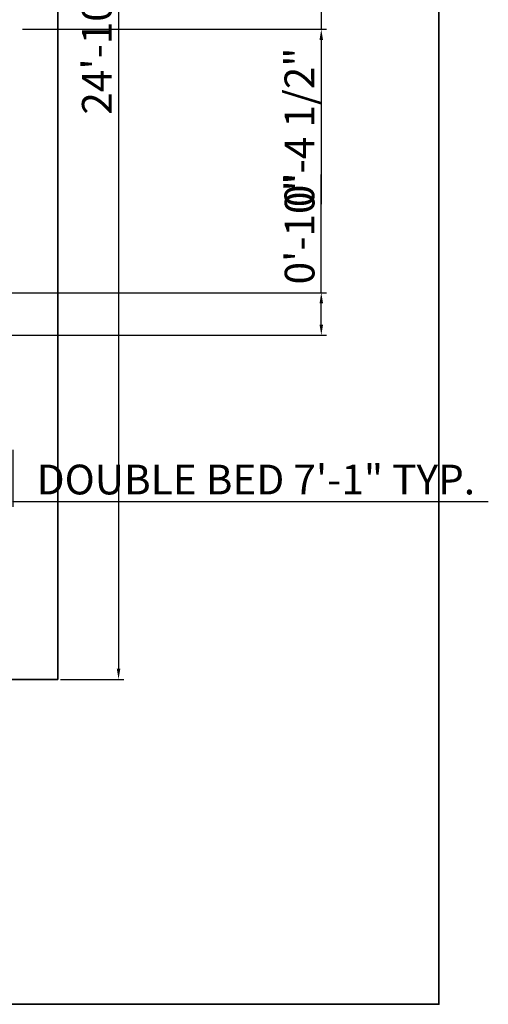
# Model space of a CAD drawing. Units: inches. Extents: x 1484 to 2008, y 1843 to 2590.
# Tile 10 of 21: x 1891 to 2001, y 1843 to 2075. Entities that reach past the tile are written whole.
import ezdxf

# ---------------------------------------------------------------- set-up
doc = ezdxf.new("R2010")
doc.units = ezdxf.units.IN
for name, color, linetype, lineweight in [('A-ANNO-DIMS', 2, 'Continuous', 18), ('A-ANNO-TTLB', 7, 'Continuous', 35), ('A-WALL', 7, 'Continuous', 35)]:
    doc.layers.add(name, color=color, linetype=linetype, lineweight=lineweight)
doc.styles.get("Standard").update_dxf_attribs({"font": 'arial.ttf'})
doc.dimstyles.new('ISO-25', dxfattribs={"dimtxt": 7, "dimasz": 2.5, "dimexe": 1.25, "dimexo": 0.625, "dimtad": 1, "dimdec": 0, "dimlunit": 3, "dimtxsty": 'Standard', "dimcen": 2.5, "dimadec": 0, "dimazin": 0, "dimtfac": 1, "dimtdec": 0, "dimtmove": 0, "dimatfit": 3, "dimfxl": 1, "dimarcsym": 0})

# ---------------------------------------------------------------- blocks, each defined once
blk = doc.blocks.new('*D3')
at = {"layer": 'A-ANNO-DIMS', "color": 0, "lineweight": -2, "transparency": 16777216}
for p, q in [((1900.54, 2217.3), (1915.42, 2217.3)), ((1914.17, 2214.8), (1914.17, 1922.3)), ((1900.54, 1919.8), (1915.42, 1919.8))]:
    blk.add_line(p, q, dxfattribs=at)
at = {"layer": 'A-ANNO-DIMS', "color": 0, "transparency": 16777216}
for points in [[(1913.75, 2214.8), (1914.58, 2214.8), (1914.17, 2217.3)], [(1913.75, 1922.3), (1914.58, 1922.3), (1914.17, 1919.8)]]:
    blk.add_solid(points, dxfattribs=at)
at = {"layer": 'Defpoints', "color": 0, "transparency": 16777216}
for p in [(1899.92, 2217.3), (1899.92, 1919.8), (1914.17, 1919.8)]:
    blk.add_point(p, dxfattribs=at)
at = {"layer": 'A-ANNO-DIMS', "color": 0, "transparency": 16777216, "insert": (1909.97, 2068.55), "char_height": 7, "attachment_point": 5, "rotation": 90}
blk.add_mtext('24\'-10"', dxfattribs=at)
blk = doc.blocks.new('*D9')
at = {"layer": 'A-ANNO-DIMS', "color": 0, "lineweight": -2, "transparency": 16777216}
for p, q in [((1804.29, 1973.81), (1804.29, 1960.43)), ((1889.31, 1973.81), (1889.31, 1960.43)), ((1806.79, 1961.68), (1886.81, 1961.68)), ((1889.31, 1961.68), (2001.13, 1961.68))]:
    blk.add_line(p, q, dxfattribs=at)
at = {"layer": 'A-ANNO-DIMS', "color": 0, "transparency": 16777216}
for points in [[(1806.79, 1962.1), (1806.79, 1961.26), (1804.29, 1961.68)], [(1886.81, 1962.1), (1886.81, 1961.26), (1889.31, 1961.68)]]:
    blk.add_solid(points, dxfattribs=at)
at = {"layer": 'Defpoints', "color": 0, "transparency": 16777216}
for p in [(1804.29, 1974.43), (1889.31, 1974.43), (1889.31, 1961.68)]:
    blk.add_point(p, dxfattribs=at)
at = {"layer": 'A-ANNO-DIMS', "color": 0, "transparency": 16777216, "insert": (1946.47, 1965.93), "char_height": 7, "attachment_point": 5}
blk.add_mtext('DOUBLE BED 7\'-1" TYP.', dxfattribs=at)
blk = doc.blocks.new('*D32')
at = {"layer": 'A-ANNO-DIMS', "color": 0, "lineweight": -2, "transparency": 16777216}
for p, q in [((1961.85, 2010.8), (1961.85, 2038.6)), ((1648.54, 2010.8), (1963.1, 2010.8)), ((1961.85, 2003.3), (1961.85, 2008.3)), ((1648.54, 2000.8), (1963.1, 2000.8))]:
    blk.add_line(p, q, dxfattribs=at)
at = {"layer": 'A-ANNO-DIMS', "color": 0, "transparency": 16777216}
for points in [[(1961.44, 2008.3), (1962.27, 2008.3), (1961.85, 2010.8)], [(1961.44, 2003.3), (1962.27, 2003.3), (1961.85, 2000.8)]]:
    blk.add_solid(points, dxfattribs=at)
at = {"layer": 'Defpoints', "color": 0, "transparency": 16777216}
for p in [(1647.92, 2010.8), (1961.85, 2010.8), (1647.92, 2000.8)]:
    blk.add_point(p, dxfattribs=at)
at = {"layer": 'A-ANNO-DIMS', "color": 0, "transparency": 16777216, "insert": (1957.66, 2025.95), "char_height": 7, "attachment_point": 5, "rotation": 90}
blk.add_mtext('0\'-10"', dxfattribs=at)
blk = doc.blocks.new('*D41')
at = {"layer": 'A-ANNO-DIMS', "color": 0, "lineweight": -2, "transparency": 16777216}
for p, q in [((1961.85, 2079.8), (1961.85, 2082.3)), ((1891.54, 2077.3), (1963.1, 2077.3)), ((1961.85, 2077.3), (1961.85, 2072.8)), ((1891.54, 2072.8), (1963.1, 2072.8)), ((1961.85, 2070.3), (1961.85, 2031.63))]:
    blk.add_line(p, q, dxfattribs=at)
at = {"layer": 'A-ANNO-DIMS', "color": 0, "transparency": 16777216}
for points in [[(1961.44, 2079.8), (1962.27, 2079.8), (1961.85, 2077.3)], [(1961.44, 2070.3), (1962.27, 2070.3), (1961.85, 2072.8)]]:
    blk.add_solid(points, dxfattribs=at)
at = {"layer": 'Defpoints', "color": 0, "transparency": 16777216}
for p in [(1890.92, 2077.3), (1890.92, 2072.8), (1961.85, 2072.8)]:
    blk.add_point(p, dxfattribs=at)
at = {"layer": 'A-ANNO-DIMS', "color": 0, "transparency": 16777216, "insert": (1957.61, 2049.72), "char_height": 7, "attachment_point": 5, "rotation": 90}
blk.add_mtext('0\'-4 1/2"', dxfattribs=at)

msp = doc.modelspace()

# ---------------------------------------------------------------- linework, layer by layer
at = {"layer": 'A-ANNO-TTLB'}
msp.add_lwpolyline([(1484.04, 2590.09), (1989.53, 2590.09), (1989.53, 1843.34), (1484.04, 1843.34)], close=True, dxfattribs=at)
at = {"layer": 'A-WALL'}
for p in [(1899.92, 2217.3), (1686.99, 1919.8)]:
    msp.add_line(p, (1899.92, 1919.8), dxfattribs=at)

# ---------------------------------------------------------------- dimensions: what is measured, and where the dimension line sits
at = {"layer": 'A-ANNO-DIMS'}
for base, p1, p2, override, picture, middle in [((1914.166081, 1919.80284398), (1899.91964371, 2217.30284398), (1899.91964371, 1919.80284398), {"dimclrd": 0, "dimclre": 0, "dimclrt": 0}, '*D3', (1909.96707009, 2068.55284398)), ((1961.85, 2072.8), (1890.92, 2077.3), (1890.92, 2072.8), {"dimdec": 1, "dimlfac": 1, "dimrnd": 0, "dimzin": 1, "dimdsep": 46, "dimlunit": 4, "dimfrac": 2}, '*D41', (1957.61, 2049.72)), ((1961.85, 2010.8), (1647.92, 2000.8), (1647.92, 2010.8), {"dimdec": 1, "dimlfac": 1, "dimrnd": 0, "dimzin": 1, "dimdsep": 46, "dimlunit": 4, "dimfrac": 2}, '*D32', (1957.66, 2025.95))]:
    dim = msp.add_linear_dim(base=base, p1=p1, p2=p2, angle=90, dimstyle='ISO-25', override=override, dxfattribs=at)
    dim.commit()
    dim.dimension.update_dxf_attribs({"geometry": picture, "text_midpoint": middle})
dim = msp.add_linear_dim(base=(1889.31, 1961.68), p1=(1804.29, 1974.43), p2=(1889.31, 1974.43), text='DOUBLE BED <> TYP.', dimstyle='ISO-25', override={"dimdec": 1, "dimlfac": 1, "dimrnd": 0, "dimzin": 1, "dimdsep": 46, "dimlunit": 4, "dimfrac": 2}, dxfattribs=at)
dim.commit()
dim.dimension.update_dxf_attribs({"geometry": '*D9', "text_midpoint": (1946.47, 1965.93)})

doc.saveas('drawing.dxf')
